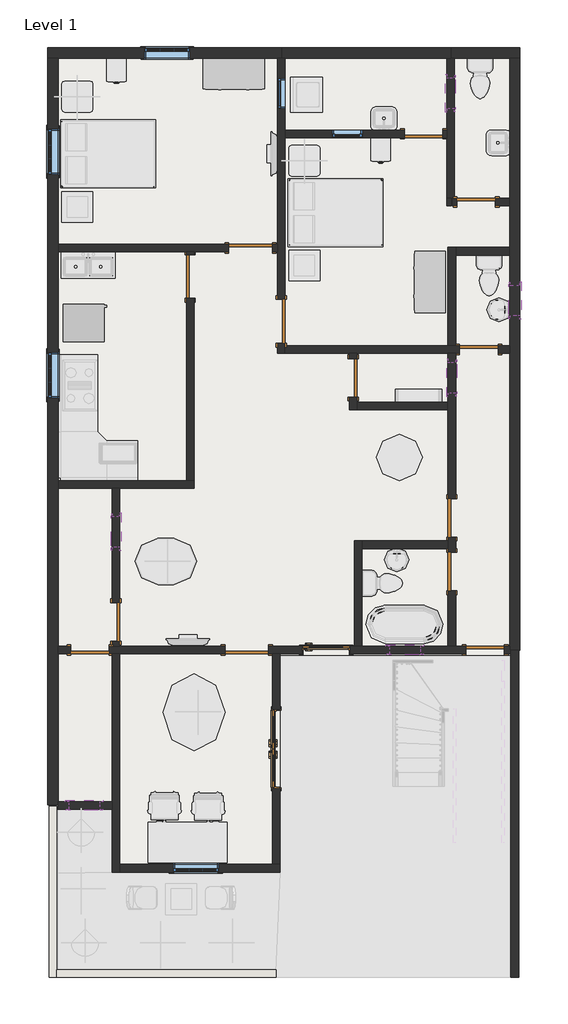
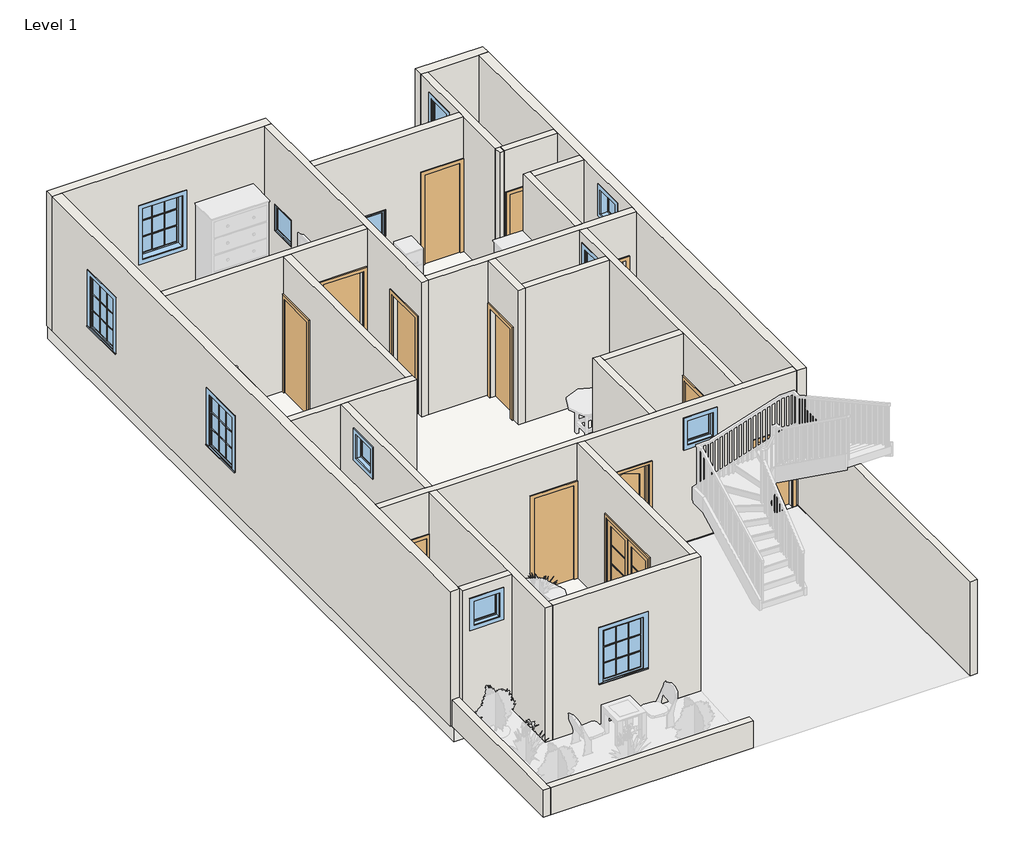
# One storey, part 1 of 3: 30 walls, 15 doors, 12 windows, 1 slab.
# Revit data of these elements (continued)
# Element 47 (IfcWindow, "Casement 3x3 with Trim : 36\" x 48\"") (continued)
#   Materials on its faces: "Sash", "Glass", "Trim"
# Element 48 (IfcWindow, "Casement 3x3 with Trim : 36\" x 48\"")
#   Mark = "2"
#   Phase Created = New Construction
#   Materials on its faces: "Sash", "Glass", "Trim"
# Element 49 (IfcWindow, "Casement 3x3 with Trim : 36\" x 48\"")
#   Mark = "3"
#   Phase Created = New Construction
#   Materials on its faces: "Sash", "Glass", "Trim"
# Element 50 (IfcWindow, "Casement 3x3 with Trim : 36\" x 48\"")
#   Mark = "4"
#   Phase Created = New Construction
#   Materials on its faces: "Sash", "Glass", "Trim"
# Element 51 (IfcWindow, "Fixed : 24\" x 24\"")
#   Mark = "5"
#   Phase Created = New Construction
#   Materials on its faces: "Sash", "Glass"
# Element 52 (IfcWindow, "Fixed : 24\" x 24\"")
#   Mark = "6"
#   Phase Created = New Construction
#   Materials on its faces: "Sash", "Glass"
# Element 53 (IfcWindow, "Transom with Trim : 24\" x 24\"")
#   Mark = "7"
#   Phase Created = New Construction
#   Materials on its faces: "Sash", "Trim", "Glass"
# Element 54 (IfcWindow, "Transom with Trim : 24\" x 24\"")
#   Mark = "8"
#   Phase Created = New Construction
#   Materials on its faces: "Sash", "Trim", "Glass"
# Element 55 (IfcWindow, "Transom with Trim : 24\" x 24\"")
#   Mark = "10"
#   Phase Created = New Construction
#   Materials on its faces: "Sash", "Trim", "Glass"
# Element 56 (IfcWindow, "Transom with Trim : 24\" x 24\"")
#   Mark = "11"
#   Phase Created = New Construction
#   Materials on its faces: "Sash", "Trim", "Glass"
# Element 57 (IfcWindow, "Transom with Trim : 24\" x 24\"")
#   Mark = "12"
#   Phase Created = New Construction
#   Materials on its faces: "Sash", "Trim", "Glass"
# Element 58 (IfcWindow, "Transom with Trim : 24\" x 24\"")
#   Mark = "9"
#   Phase Created = New Construction
#   Materials on its faces: "Sash", "Trim", "Glass"
# Materials
#   "Cherry": class "Wood", colour RGB 226 177 128, transparency 0, Description = "Prunus Serotina", Cost = 0
#   "Glass": class "Glass", colour RGB 0 128 192, transparency 0.75, Description = "Soda Lime Glass", Cost = 0
#   "Aluminum": class "Metal", colour RGB 247 247 247, transparency 0, Description = "Aluminum 6061", Cost = 0
#   "Door - Panel": class "Wood", colour RGB 210 159 95, transparency 0
#   "Door - Frame": colour RGB 118 70 51, transparency 0
#   "Birch": class "Wood", colour RGB 224 178 126, transparency 0, Description = "Betula Alleghaniensis", Cost = 0
#   "Brick, Common": class "Masonry", colour RGB 170 98 104, transparency 0, Description = "Common brick", Cost = 0
#   "Sash": class "Wood", colour RGB 224 178 126, transparency 0
#   "Trim": class "Wood", colour RGB 224 178 126, transparency 0
#   "Default Floor": colour RGB 128 128 128, transparency 0
# Room at (-10184.808, 4271.72) mm, phase "New Construction", upper level "Level 1", upper offset 10' - 0", lower offset 0' - 0"
#   Number = "11"
#   Name = "HALL"
# Room at (-11699.715, -1417.83) mm, phase "New Construction", upper level "Level 1", upper offset 10' - 0", lower offset 0' - 0"
#   Number = "12"
#   Name = "DRAWING"
# Room at (-12804.692, -4509.446) mm, phase "New Construction", upper level "Level 1", upper offset 10' - 0", lower offset 0' - 0"
#   Number = "13"
#   Name = "LAWN AREA"
# Room at (-7563.728, -3247.29) mm, phase "New Construction", upper level "Level 1", upper offset 10' - 0", lower offset 0' - 0"
#   Number = "14"
#   Name = "PORCH"
# Room at (-12272.093, 11189.824) mm, phase "New Construction", upper level "Level 1", upper offset 10' - 0", lower offset 0' - 0"
#   Number = "1"
#   Name = "BEDROOM"
# Room at (-8472.06, 12045.58) mm, phase "New Construction", upper level "Level 1", upper offset 10' - 0", lower offset 0' - 0"
#   Number = "2"
#   Name = "OPEN"
# Room at (-6012.896, 11437.619) mm, phase "New Construction", upper level "Level 1", upper offset 10' - 0", lower offset 0' - 0"
#   Number = "3"
#   Name = "TOILET"
# Room at (-8472.06, 9148.886) mm, phase "New Construction", upper level "Level 1", upper offset 10' - 0", lower offset 0' - 0"
#   Number = "4"
#   Name = "BEDROOM"
# Room at (-5998.39, 8076.495) mm, phase "New Construction", upper level "Level 1", upper offset 10' - 0", lower offset 0' - 0"
#   Number = "5"
#   Name = "TOILET"
# Room at (-5943.201, 5096.316) mm, phase "New Construction", upper level "Level 1", upper offset 10' - 0", lower offset 0' - 0"
#   Number = "6"
#   Name = "UTILITY"
# Room at (-7563.728, 1798.385) mm, phase "New Construction", upper level "Level 1", upper offset 10' - 0", lower offset 0' - 0"
#   Number = "7"
#   Name = "BATH"
# Room at (-13280.903, 6172.085) mm, phase "New Construction", upper level "Level 1", upper offset 10' - 0", lower offset 0' - 0"
#   Number = "8"
#   Name = "KITCHEN"
# Room at (-7563.728, 6172.085) mm, phase "New Construction", upper level "Level 1", upper offset 10' - 0", lower offset 0' - 0"
#   Number = "9"
#   Name = "STORE"
# Room at (-13987.638, -1124.156) mm, phase "New Construction", upper level "Level 1", upper offset 10' - 0", lower offset 0' - 0"
#   Number = "10"
